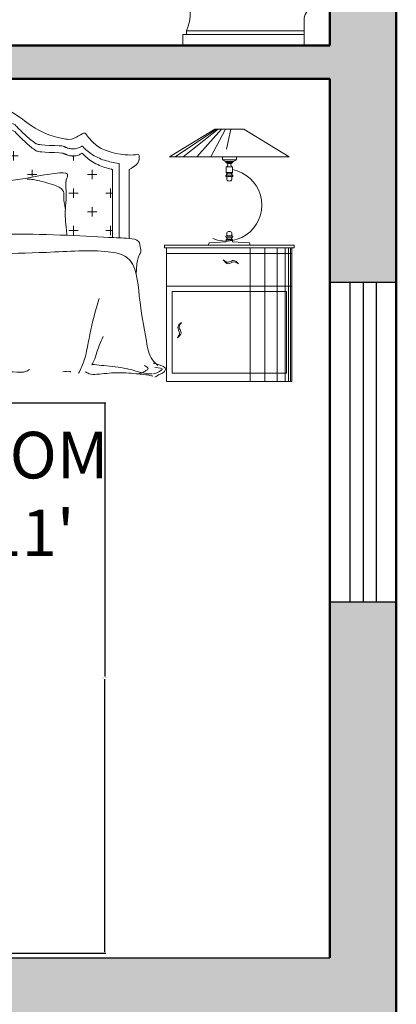
# Model space of a CAD drawing. Units: inches. Extents: x 1771 to 3025, y 319 to 889.
# Tile 17 of 35: x 2505 to 2561, y 473 to 621. Entities that reach past the tile are written whole.
import ezdxf

# ---------------------------------------------------------------- set-up
doc = ezdxf.new("R2010")
doc.units = ezdxf.units.IN
doc.header["$MEASUREMENT"] = 0
for name, color, linetype, lineweight in [('A-ANNO-DIMS', 2, 'Continuous', 18), ('A-AREA-IDEN', 241, 'Continuous', 25), ('A-FLOR-FIXT', 8, 'Continuous', 18), ('A-FLOR-STRS', 7, 'Continuous', 25), ('A-FURN', 8, 'Continuous', 18), ('A-GLAZ', 40, 'Continuous', 25), ('A-WALL', 7, 'Continuous', 50), ('A-WALL-PATT', 254, 'Continuous', 13)]:
    doc.layers.add(name, color=color, linetype=linetype, lineweight=lineweight)
doc.styles.get("Standard").update_dxf_attribs({"font": 'arial.ttf'})
doc.dimstyles.get("Standard").update_dxf_attribs({"dimtxt": 0.18, "dimasz": 0.18, "dimexe": 0.18, "dimexo": 0.0625, "dimgap": 0.09, "dimtad": 0, "dimtih": 1, "dimtoh": 1, "dimdec": 4, "dimzin": 0, "dimdsep": 46, "dimtxsty": 'Standard', "dimcen": 0.09, "dimadec": 0, "dimazin": 0, "dimtfac": 1, "dimtdec": 4, "dimtofl": 0, "dimtmove": 0, "dimatfit": 3, "dimfxl": 1, "dimtolj": 1, "dimtzin": 0, "dimarcsym": 0})

# ---------------------------------------------------------------- blocks, each defined once
blk = doc.blocks.new('A$C3908634B')
at = {"ltscale": 5}
for p, q in [((1200.2, 1046.3), (1218.1, 1046.3)), ((1176, 731), (1176, 731.7))]:
    blk.add_line(p, q, dxfattribs=at)
for p, q in [((1253.9, 945.1), (1253.9, 978.5)), ((1100.9, 962.2), (1134.6, 962.2)), ((1117.6, 945.1), (1117.6, 967.5)), ((1236.9, 962.2), (1271, 962.2)), ((184.3, 923.4), (19, 823.1)), ((237.5, 923.4), (184.3, 923.4)), ((190.2, 923.4), (237.5, 923.4)), ((231.9, 923.4), (247.3, 851.1)), ((284.7, 923.4), (237.5, 923.4)), ((237.5, 923.4), (290.6, 923.4)), ((251.7, 923.4), (305.7, 823.1)), ((266, 923.4), (356.4, 823.1)), ((278.7, 923.4), (406.8, 823.1)), ((284.7, 923.4), (436.3, 823.1)), ((290.6, 923.4), (456, 823.1)), ((1049.4, 876.9), (1049.4, 911)), ((1185.7, 876.9), (1185.7, 911)), ((1322.1, 876.9), (1322.1, 911)), ((2198.9, 923.4), (2033.5, 823.1)), ((2204.8, 923.4), (2053.3, 823.1)), ((2210.8, 923.4), (2082.7, 823.1)), ((2223.5, 923.4), (2133.1, 823.1)), ((2237.8, 923.4), (2183.8, 823.1)), ((2252, 923.4), (2198.9, 923.4)), ((2204.8, 923.4), (2252, 923.4)), ((2257.6, 923.4), (2242.2, 851.1)), ((2299.3, 923.4), (2252, 923.4)), ((2252, 923.4), (2305.2, 923.4)), ((2305.2, 923.4), (2470.5, 823.1)), ((1032.3, 894), (1066.4, 894)), ((1168.7, 894), (1202.8, 894)), ((1305.1, 894), (1339.1, 894)), ((940, 808.8), (940, 842.9)), ((1117.6, 808.8), (1117.6, 842.9)), ((1253.9, 808.8), (1253.9, 842.9)), ((1462.5, 808.8), (1462.5, 842.9)), ((237.5, 823.1), (19, 823.1)), ((212, 823.1), (212, 811.7)), ((212, 811.7), (223, 805.4)), ((212, 811.7), (237.5, 811.7)), ((223, 805.4), (224.6, 801.4)), ((223, 805.4), (237.5, 805.4)), ((250.4, 801.4), (224.6, 801.4)), ((226.9, 801.4), (228.3, 798.3)), ((228.3, 798.3), (237.5, 798.3)), ((228.3, 798.3), (231.3, 797.6)), ((231.3, 797.6), (232, 794.9)), ((231.9, 793.9), (231.6, 792.6)), ((232, 794.9), (231.9, 793.9)), ((237.5, 823.1), (456, 823.1)), ((263, 811.7), (237.5, 811.7)), ((252, 805.4), (237.5, 805.4)), ((246.7, 798.3), (237.5, 798.3)), ((243.7, 797.6), (243, 794.9)), ((243, 794.9), (243.1, 793.9)), ((243.1, 793.9), (243.4, 792.6)), ((246.7, 798.3), (243.7, 797.6)), ((248.1, 801.4), (246.7, 798.3)), ((252, 805.4), (250.4, 801.4)), ((263, 811.7), (252, 805.4)), ((263, 823.1), (263, 811.7)), ((621.3, 798.8), (621.3, 526)), ((741.7, 808.8), (741.7, 821.7)), ((746.2, 825.8), (758.8, 825.8)), ((922.9, 825.8), (957, 825.8)), ((1100.5, 825.8), (1134.6, 825.8)), ((1236.9, 825.8), (1271, 825.8)), ((1373.2, 825.8), (1479.5, 825.8)), ((1681.3, 808.8), (1681.3, 825.6)), ((1848.6, 798.8), (1848.6, 526.2)), ((2252, 823.1), (2033.5, 823.1)), ((2226.5, 823.1), (2226.5, 811.7)), ((2226.5, 811.7), (2237.6, 805.4)), ((2226.5, 811.7), (2252, 811.7)), ((2237.6, 805.4), (2239.1, 801.4)), ((2237.6, 805.4), (2252, 805.4)), ((2239.1, 801.4), (2264.9, 801.4)), ((2241.4, 801.4), (2242.8, 798.3)), ((2242.8, 798.3), (2245.8, 797.6)), ((2242.8, 798.3), (2252, 798.3)), ((2245.8, 797.6), (2246.5, 794.9)), ((2246.4, 793.9), (2246.1, 792.6)), ((2246.5, 794.9), (2246.4, 793.9)), ((2252, 823.1), (2470.5, 823.1)), ((2277.6, 811.7), (2252, 811.7)), ((2266.5, 805.4), (2252, 805.4)), ((2261.2, 798.3), (2252, 798.3)), ((2258.2, 797.6), (2257.6, 794.9)), ((2257.6, 794.9), (2257.6, 793.9)), ((2257.6, 793.9), (2257.9, 792.6)), ((2261.2, 798.3), (2258.2, 797.6)), ((2262.6, 801.4), (2261.2, 798.3)), ((2266.5, 805.4), (2264.9, 801.4)), ((2277.6, 811.7), (2266.5, 805.4)), ((2277.6, 823.1), (2277.6, 811.7)), ((227.8, 786.4), (226.2, 785.6)), ((226.2, 785.6), (226.2, 765)), ((226.2, 785.6), (248.8, 785.6)), ((226.2, 765), (227.6, 764.2)), ((226.2, 765), (237.5, 765)), ((227.4, 757.9), (227.1, 757.2)), ((227.1, 757.2), (227.3, 756.6)), ((227.3, 756.6), (227.8, 755.9)), ((227.7, 758.5), (227.4, 757.9)), ((227.6, 764.2), (228.5, 763.3)), ((228.6, 758.7), (227.7, 758.5)), ((230.2, 788), (227.8, 786.4)), ((228.5, 763.3), (229.4, 762.5)), ((228.5, 763.3), (237.5, 763.3)), ((229.4, 759.1), (228.6, 758.7)), ((229.4, 762.5), (230, 761.4)), ((229.8, 759.5), (229.4, 759.1)), ((230.1, 760.2), (229.8, 759.5)), ((230, 761.4), (230.1, 760.2)), ((231.1, 790.5), (230.2, 788)), ((231.5, 791.1), (231.1, 790.5)), ((231.6, 792.6), (231.5, 791.9)), ((231.5, 791.9), (231.5, 791.1)), ((248.8, 765), (237.5, 765)), ((246.5, 763.3), (237.5, 763.3)), ((243.4, 792.6), (243.4, 791.9)), ((243.4, 791.9), (243.4, 791.1)), ((243.4, 791.1), (243.9, 790.5)), ((243.9, 790.5), (244.8, 788)), ((244.8, 788), (247.2, 786.4)), ((245, 761.4), (244.9, 760.2)), ((244.9, 760.2), (245.2, 759.5)), ((245.6, 762.5), (245, 761.4)), ((245.2, 759.5), (245.6, 759.1)), ((246.5, 763.3), (245.6, 762.5)), ((245.6, 759.1), (246.4, 758.7)), ((246.4, 758.7), (247.3, 758.5)), ((247.4, 764.2), (246.5, 763.3)), ((247.2, 786.4), (248.8, 785.6)), ((247.7, 756.6), (247.2, 755.9)), ((247.3, 758.5), (247.6, 757.9)), ((248.8, 765), (247.4, 764.2)), ((247.6, 757.9), (247.9, 757.2)), ((247.9, 757.2), (247.7, 756.6)), ((248.8, 785.6), (248.8, 765)), ((645.8, 776.5), (645.8, 527)), ((656.5, 757.6), (690.6, 757.6)), ((673.5, 740.6), (673.5, 774.7)), ((792.9, 757.6), (827, 757.6)), ((809.9, 740.6), (809.9, 774.7)), ((1032.3, 757.6), (1066.4, 757.6)), ((1049.4, 740.6), (1049.4, 774.7)), ((1168.7, 757.6), (1202.8, 757.6)), ((1185.7, 740.6), (1185.7, 774.7)), ((1305.1, 757.6), (1339.1, 757.6)), ((1322.1, 740.6), (1322.1, 774.7)), ((1513.6, 757.6), (1547.7, 757.6)), ((1530.6, 751.3), (1530.6, 774.7)), ((1732.4, 757.6), (1766.5, 757.6)), ((1749.5, 740.6), (1749.5, 774.7)), ((1824, 776.5), (1824, 527.2)), ((2242.3, 786.4), (2240.7, 785.6)), ((2240.7, 785.6), (2240.7, 765)), ((2263.3, 785.6), (2240.7, 785.6)), ((2240.7, 765), (2242.1, 764.2)), ((2240.7, 765), (2252, 765)), ((2241.9, 757.9), (2241.7, 757.2)), ((2241.7, 757.2), (2241.8, 756.6)), ((2241.8, 756.6), (2242.3, 755.9)), ((2242.2, 758.5), (2241.9, 757.9)), ((2242.1, 764.2), (2243, 763.3)), ((2243.1, 758.7), (2242.2, 758.5)), ((2244.7, 788), (2242.3, 786.4)), ((2243, 763.3), (2243.9, 762.5)), ((2243, 763.3), (2252, 763.3)), ((2243.9, 759.1), (2243.1, 758.7)), ((2243.9, 762.5), (2244.6, 761.4)), ((2244.3, 759.5), (2243.9, 759.1)), ((2244.6, 760.2), (2244.3, 759.5)), ((2244.6, 761.4), (2244.6, 760.2)), ((2245.6, 790.5), (2244.7, 788)), ((2246.1, 791.1), (2245.6, 790.5)), ((2246.1, 792.6), (2246.1, 791.9)), ((2246.1, 791.9), (2246.1, 791.1)), ((2263.3, 765), (2252, 765)), ((2261.1, 763.3), (2252, 763.3)), ((2257.9, 792.6), (2258, 791.9)), ((2258, 791.9), (2258, 791.1)), ((2258, 791.1), (2258.4, 790.5)), ((2258.4, 790.5), (2259.4, 788)), ((2259.4, 788), (2261.7, 786.4)), ((2259.5, 761.4), (2259.4, 760.2)), ((2259.4, 760.2), (2259.7, 759.5)), ((2260.1, 762.5), (2259.5, 761.4)), ((2259.7, 759.5), (2260.1, 759.1)), ((2261.1, 763.3), (2260.1, 762.5)), ((2260.1, 759.1), (2260.9, 758.7)), ((2260.9, 758.7), (2261.8, 758.5)), ((2261.9, 764.2), (2261.1, 763.3)), ((2261.7, 786.4), (2263.3, 785.6)), ((2261.8, 758.5), (2262.2, 757.9)), ((2262.2, 756.6), (2261.8, 755.9)), ((2263.3, 765), (2261.9, 764.2)), ((2262.2, 757.9), (2262.4, 757.2)), ((2262.4, 757.2), (2262.2, 756.6)), ((2263.3, 785.6), (2263.3, 765)), ((224.8, 753.5), (224.7, 752.9)), ((224.7, 752.9), (224.8, 752.1)), ((225.3, 753.9), (224.8, 753.5)), ((224.8, 752.1), (225.2, 751.4)), ((225.2, 751.4), (225.6, 750.9)), ((225.7, 754.3), (225.3, 753.9)), ((225.6, 750.9), (228.1, 750.2)), ((226.3, 754.6), (225.7, 754.3)), ((227, 754.7), (226.3, 754.6)), ((227.9, 754.7), (227, 754.7)), ((227.8, 755.9), (228.9, 755.2)), ((228.9, 755.2), (227.9, 754.7)), ((228.1, 750.2), (229.9, 750)), ((228.9, 755.2), (237.5, 755.2)), ((229.9, 750), (232.4, 750.2)), ((232.4, 750.2), (237.5, 750.2)), ((246.1, 755.2), (237.5, 755.2)), ((242.6, 750.2), (237.5, 750.2)), ((245.1, 750), (242.6, 750.2)), ((246.9, 750.2), (245.1, 750)), ((247.2, 755.9), (246.1, 755.2)), ((246.1, 755.2), (247.1, 754.7)), ((249.4, 750.9), (246.9, 750.2)), ((247.1, 754.7), (248, 754.7)), ((248, 754.7), (248.7, 754.6)), ((248.7, 754.6), (249.3, 754.3)), ((249.3, 754.3), (249.7, 753.9)), ((249.8, 751.4), (249.4, 750.9)), ((249.7, 753.9), (250.2, 753.5)), ((250.2, 752.1), (249.8, 751.4)), ((250.2, 753.5), (250.3, 752.9)), ((250.3, 752.9), (250.2, 752.1)), ((2239.4, 753.5), (2239.2, 752.9)), ((2239.2, 752.9), (2239.3, 752.1)), ((2239.3, 752.1), (2239.7, 751.4)), ((2239.9, 753.9), (2239.4, 753.5)), ((2239.7, 751.4), (2240.2, 750.9)), ((2240.3, 754.3), (2239.9, 753.9)), ((2240.2, 750.9), (2242.6, 750.2)), ((2240.8, 754.6), (2240.3, 754.3)), ((2241.5, 754.7), (2240.8, 754.6)), ((2242.4, 754.7), (2241.5, 754.7)), ((2242.3, 755.9), (2243.4, 755.2)), ((2243.4, 755.2), (2242.4, 754.7)), ((2242.6, 750.2), (2244.4, 750)), ((2243.4, 755.2), (2252, 755.2)), ((2244.4, 750), (2246.9, 750.2)), ((2246.9, 750.2), (2252, 750.2)), ((2260.7, 755.2), (2252, 755.2)), ((2257.1, 750.2), (2252, 750.2)), ((2259.6, 750), (2257.1, 750.2)), ((2261.5, 750.2), (2259.6, 750)), ((2261.8, 755.9), (2260.7, 755.2)), ((2260.7, 755.2), (2261.6, 754.7)), ((2263.9, 750.9), (2261.5, 750.2)), ((2261.6, 754.7), (2262.5, 754.7)), ((2262.5, 754.7), (2263.2, 754.6)), ((2263.2, 754.6), (2263.8, 754.3)), ((2263.8, 754.3), (2264.2, 753.9)), ((2264.3, 751.4), (2263.9, 750.9)), ((2264.2, 753.9), (2264.7, 753.5)), ((2264.7, 752.1), (2264.3, 751.4)), ((2264.7, 753.5), (2264.8, 752.9)), ((2264.8, 752.9), (2264.7, 752.1)), ((724.7, 689.4), (758.8, 689.4)), ((741.7, 672.4), (741.7, 706.5)), ((922.9, 689.4), (957, 689.4)), ((940, 672.4), (940, 706.5)), ((1100.5, 689.4), (1134.6, 689.4)), ((1117.6, 672.4), (1117.6, 706.5)), ((1664.3, 689.4), (1698.3, 689.4)), ((1681.3, 672.4), (1681.3, 706.5)), ((1800.6, 689.4), (1824, 689.4)), ((1817.7, 672.4), (1817.7, 706.5)), ((656.5, 621.3), (690.6, 621.3)), ((673.5, 604.2), (673.5, 638.3)), ((792.9, 621.3), (823.2, 621.3)), ((809.9, 604.2), (809.9, 638.3)), ((1732.4, 621.3), (1766.5, 621.3)), ((1749.5, 604.2), (1749.5, 638.3)), ((724.7, 553.1), (758.8, 553.1)), ((741.7, 536), (741.7, 570.1)), ((1664.3, 553.1), (1698.3, 553.1)), ((1681.3, 536), (1681.3, 570.1)), ((1800.6, 553.1), (1824, 553.1)), ((1817.7, 536), (1817.7, 570.1)), ((164, 507.9), (161.1, 499.5)), ((164, 507.9), (226.2, 512.1)), ((224.7, 530.9), (224.8, 531.7)), ((224.8, 530.3), (224.7, 530.9)), ((224.8, 531.7), (225.2, 532.4)), ((225.3, 529.9), (224.8, 530.3)), ((225.2, 532.4), (225.6, 532.9)), ((225.7, 529.5), (225.3, 529.9)), ((225.6, 532.9), (228.1, 533.6)), ((226.3, 529.2), (225.7, 529.5)), ((226.2, 518.8), (227.6, 519.6)), ((226.2, 512.1), (226.2, 518.8)), ((226.2, 518.8), (237.5, 518.8)), ((227, 529.1), (226.3, 529.2)), ((227.9, 529.1), (227, 529.1)), ((227.1, 526.6), (227.3, 527.2)), ((227.4, 525.9), (227.1, 526.6)), ((227.3, 527.2), (227.8, 527.9)), ((227.7, 525.3), (227.4, 525.9)), ((227.6, 519.6), (228.5, 520.5)), ((228.6, 525.1), (227.7, 525.3)), ((227.8, 527.9), (228.9, 528.6)), ((228.9, 528.6), (227.9, 529.1)), ((228.1, 533.6), (229.9, 533.8)), ((228.5, 520.5), (229.4, 521.3)), ((229.4, 524.7), (228.6, 525.1)), ((228.9, 528.6), (237.5, 528.6)), ((229.8, 524.3), (229.4, 524.7)), ((229.4, 521.3), (230, 522.4)), ((229.4, 521.3), (237.5, 521.3)), ((230.1, 523.6), (229.8, 524.3)), ((230, 522.4), (230.1, 523.6)), ((230.3, 533.8), (237.5, 533.6)), ((242.6, 533.6), (237.5, 533.6)), ((246.1, 528.6), (237.5, 528.6)), ((245.6, 521.3), (237.5, 521.3)), ((248.8, 518.8), (237.5, 518.8)), ((245.1, 533.8), (242.6, 533.6)), ((244.9, 523.6), (245.2, 524.3)), ((245, 522.4), (244.9, 523.6)), ((245.6, 521.3), (245, 522.4)), ((246.9, 533.6), (245.1, 533.8)), ((245.2, 524.3), (245.6, 524.7)), ((245.6, 524.7), (246.4, 525.1)), ((246.5, 520.5), (245.6, 521.3)), ((246.1, 528.6), (247.1, 529.1)), ((247.2, 527.9), (246.1, 528.6)), ((246.4, 525.1), (247.3, 525.3)), ((247.4, 519.6), (246.5, 520.5)), ((249.4, 532.9), (246.9, 533.6)), ((247.1, 529.1), (248, 529.1)), ((247.7, 527.2), (247.2, 527.9)), ((247.3, 525.3), (247.6, 525.9)), ((248.8, 518.8), (247.4, 519.6)), ((247.6, 525.9), (247.9, 526.6)), ((247.9, 526.6), (247.7, 527.2)), ((248, 529.1), (248.7, 529.2)), ((248.7, 529.2), (249.3, 529.5)), ((248.8, 512.1), (248.8, 518.8)), ((311, 507.9), (248.8, 512.1)), ((249.3, 529.5), (249.7, 529.9)), ((249.8, 532.4), (249.4, 532.9)), ((249.7, 529.9), (250.2, 530.3)), ((250.2, 531.7), (249.8, 532.4)), ((250.3, 530.9), (250.2, 531.7)), ((250.2, 530.3), (250.3, 530.9)), ((311, 507.9), (315.3, 499.5)), ((2178.5, 507.9), (2174.2, 499.5)), ((2178.5, 507.9), (2240.7, 512.1)), ((2239.2, 530.9), (2239.3, 531.7)), ((2239.4, 530.3), (2239.2, 530.9)), ((2239.3, 531.7), (2239.7, 532.4)), ((2239.9, 529.9), (2239.4, 530.3)), ((2239.7, 532.4), (2240.2, 532.9)), ((2240.3, 529.5), (2239.9, 529.9)), ((2240.2, 532.9), (2242.6, 533.6)), ((2240.8, 529.2), (2240.3, 529.5)), ((2240.7, 518.8), (2242.1, 519.6)), ((2240.7, 512.1), (2240.7, 518.8)), ((2240.7, 518.8), (2252, 518.8)), ((2241.5, 529.1), (2240.8, 529.2)), ((2242.4, 529.1), (2241.5, 529.1)), ((2241.7, 526.6), (2241.8, 527.2)), ((2241.9, 525.9), (2241.7, 526.6)), ((2241.8, 527.2), (2242.3, 527.9)), ((2242.2, 525.3), (2241.9, 525.9)), ((2242.1, 519.6), (2243, 520.5)), ((2243.1, 525.1), (2242.2, 525.3)), ((2242.3, 527.9), (2243.4, 528.6)), ((2243.4, 528.6), (2242.4, 529.1)), ((2242.6, 533.6), (2244.4, 533.8)), ((2243, 520.5), (2243.9, 521.3)), ((2243.9, 524.7), (2243.1, 525.1)), ((2243.4, 528.6), (2252, 528.6)), ((2244.3, 524.3), (2243.9, 524.7)), ((2243.9, 521.3), (2244.6, 522.4)), ((2243.9, 521.3), (2252, 521.3)), ((2244.6, 523.6), (2244.3, 524.3)), ((2244.4, 533.8), (2246.9, 533.6)), ((2244.6, 522.4), (2244.6, 523.6)), ((2246.9, 533.6), (2252, 533.6)), ((2259.2, 533.8), (2252, 533.6)), ((2260.7, 528.6), (2252, 528.6)), ((2260.1, 521.3), (2252, 521.3)), ((2263.3, 518.8), (2252, 518.8)), ((2259.4, 523.6), (2259.7, 524.3)), ((2259.5, 522.4), (2259.4, 523.6)), ((2260.1, 521.3), (2259.5, 522.4)), ((2261.5, 533.6), (2259.6, 533.8)), ((2259.7, 524.3), (2260.1, 524.7)), ((2260.1, 524.7), (2260.9, 525.1)), ((2261.1, 520.5), (2260.1, 521.3)), ((2260.7, 528.6), (2261.6, 529.1)), ((2261.8, 527.9), (2260.7, 528.6)), ((2260.9, 525.1), (2261.8, 525.3)), ((2261.9, 519.6), (2261.1, 520.5)), ((2263.9, 532.9), (2261.5, 533.6)), ((2261.6, 529.1), (2262.5, 529.1)), ((2262.2, 527.2), (2261.8, 527.9)), ((2261.8, 525.3), (2262.2, 525.9)), ((2263.3, 518.8), (2261.9, 519.6)), ((2262.4, 526.6), (2262.2, 527.2)), ((2262.2, 525.9), (2262.4, 526.6)), ((2262.5, 529.1), (2263.2, 529.2)), ((2263.2, 529.2), (2263.8, 529.5)), ((2263.3, 512.1), (2263.3, 518.8)), ((2325.5, 507.9), (2263.3, 512.1)), ((2263.8, 529.5), (2264.2, 529.9)), ((2264.3, 532.4), (2263.9, 532.9)), ((2264.2, 529.9), (2264.7, 530.3)), ((2264.7, 531.7), (2264.3, 532.4)), ((2264.8, 530.9), (2264.7, 531.7)), ((2264.7, 530.3), (2264.8, 530.9)), ((2325.5, 507.9), (2328.4, 499.5)), ((475, 499.5), (0, 499.5)), ((0, 499.5), (0, 489.5)), ((475, 489.5), (0, 489.5)), ((8.7, 489.5), (8.7, 0)), ((467.1, 469.5), (8.7, 469.5)), ((14.1, 488.6), (14.1, 0)), ((21.3, 488.6), (21.3, 0)), ((33, 488.6), (33, 0)), ((62.7, 488.6), (62.7, 0)), ((107.6, 488.6), (107.6, 0)), ((161.1, 499.5), (237.5, 499.5)), ((161.6, 488.6), (161.6, 0)), ((315.3, 499.5), (237.5, 499.5)), ((467.1, 0), (467.1, 489.5)), ((475, 499.5), (475, 489.5)), ((2014.5, 499.5), (2489.5, 499.5)), ((2014.5, 499.5), (2014.5, 489.5)), ((2014.5, 489.5), (2489.5, 489.5)), ((2022.4, 0), (2022.4, 489.5)), ((2022.4, 469.5), (2480.8, 469.5)), ((2174.2, 499.5), (2252, 499.5)), ((2328.4, 499.5), (2252, 499.5)), ((2327.9, 488.6), (2327.9, 0)), ((2381.9, 488.6), (2381.9, 0)), ((2426.8, 488.6), (2426.8, 0)), ((2456.5, 488.6), (2456.5, 0)), ((2468.2, 488.6), (2468.2, 0)), ((2475.4, 488.6), (2475.4, 0)), ((2480.8, 489.5), (2480.8, 0)), ((2489.5, 499.5), (2489.5, 489.5)), ((467.1, 349.5), (8.7, 349.5)), ((28.7, 329.5), (28.7, 31.6)), ((447.1, 329.5), (28.7, 329.5)), ((447.1, 31.6), (447.1, 329.5)), ((2022.4, 349.5), (2480.8, 349.5)), ((2042.4, 329.5), (2460.8, 329.5)), ((2042.4, 31.6), (2042.4, 329.5)), ((2460.8, 329.5), (2460.8, 31.6)), ((467.1, 281.6), (467.1, 301.6)), ((2022.4, 281.6), (2022.4, 301.6)), ((8.7, 0), (467.1, 0)), ((28.7, 31.6), (447.1, 31.6)), ((2022.4, 0), (2480.8, 0)), ((2460.8, 31.6), (2042.4, 31.6))]:
    blk.add_line(p, q)
at = {"ltscale": 20}
for p, q in [((584.4, 776.7), (584.4, 523.7)), ((1885.4, 776.7), (1885.4, 524))]:
    blk.add_line(p, q, dxfattribs=at)
for centre, radius, start, end in [((1209.1, 956.2), 55.2, 80.5605, 99.4395), ((1209.1, 930.3), 55.2, 80.5605, 99.4395), ((250.5, 646.2), 131.8, 100.6234, 291.2), ((2239, 646.2), 131.8, 248.8, 79.3766), ((237.5, 743.5), 9.69, 137.7341, 270), ((237.5, 743.5), 9.69, 270, 42.2659), ((2252, 743.5), 9.69, 137.7341, 270), ((2252, 743.5), 9.69, 270, 42.2659), ((237.5, 540.3), 9.69, 90, 222.2659), ((237.5, 540.3), 9.69, 317.7341, 90), ((2252, 540.3), 9.69, 90, 222.2659), ((2252, 540.3), 9.69, 317.7341, 90)]:
    blk.add_arc(centre, radius, start, end)
for points in [[(584.4, 776.7), (563.9, 786.2), (546, 802.1), (547.3, 834.8), (564.5, 828.3), (620.6, 830.4), (706.4, 847.2), (752.1, 924.2), (778.1, 880.4), (846.1, 907.1), (1017.7, 1014.1), (1134.5, 1035.5), (1200.2, 1046.3)], [(1885.4, 776.7), (1905.9, 786.2), (1923.9, 802.1), (1922.5, 834.8), (1905.3, 828.3), (1849.2, 830.4), (1763.4, 847.2), (1717.7, 924.2), (1691.7, 880.4), (1541.2, 907.1), (1472.8, 1014.1), (1283.8, 1035.5), (1218.1, 1046.3)]]:
    blk.add_open_spline(points, degree=3, knots=[12.417853, 12.417853, 12.417853, 12.417853, 68.394536, 90.665986, 114.156853, 157.554067, 281.869614, 298.858744, 338.737111, 347.060176, 470.423438, 625.498764, 625.498764, 625.498764, 625.498764], dxfattribs=at)
for points, knots in [([(756.1, 861.8), (756.9, 861.3), (757.6, 860.9), (759.9, 859.6), (761.6, 858.7), (765.5, 856.8), (767.8, 855.8), (772.7, 854.1), (775.4, 853.3), (780.8, 852.2), (783.3, 851.8), (787.1, 851.6), (788.2, 851.5), (789.9, 851.5), (790.6, 851.5), (791.9, 851.5), (792.5, 851.5), (793.6, 851.6), (794.1, 851.6), (795.8, 851.8), (796.8, 851.9), (800.3, 852.3), (802.5, 852.8), (806.5, 853.8), (808.3, 854.3), (811.5, 855.4), (812.9, 855.9), (815.3, 856.9), (816.4, 857.4), (817.6, 857.9), (817.8, 858), (818.4, 858.2), (818.7, 858.4), (819.5, 858.7), (820, 859), (821.6, 859.7), (822.7, 860.2), (825.8, 861.7), (827.9, 862.8), (834, 866), (837.9, 868.3), (848.5, 874.9), (854.9, 879.4), (928.8, 888.8), (934.4, 893.5), (945, 903.2), (950, 908), (1000.9, 917.4), (1005.5, 922.1), (1014.4, 931), (1018.7, 935.3), (1027, 943.5), (1031.1, 947.3), (1036.9, 952.4), (1038.8, 954), (1042, 956.7), (1043.5, 957.9), (1045.8, 959.7), (1046.7, 960.3), (1048.5, 961.7), (1049.4, 962.3), (1052.1, 964.2), (1054, 965.5), (1059.7, 969.2), (1063.6, 971.5), (1074.8, 977.5), (1082.2, 980.9), (1098, 987.2), (1106.3, 990), (1123.7, 995.2), (1132.8, 997.5), (1151.5, 1001.8), (1161.1, 1003.8), (1180.5, 1007.4), (1190.2, 1009), (1200.1, 1010.7)], [328.6705, 328.6705, 328.6705, 328.6705, 329.609368, 329.609368, 331.487103, 331.487103, 333.620342, 333.620342, 335.753581, 335.753581, 337.507866, 337.507866, 338.182373, 338.182373, 338.607397, 338.607397, 338.959312, 338.959312, 339.311227, 339.311227, 340.015058, 340.015058, 341.722742, 341.722742, 343.430427, 343.430427, 345.138111, 345.138111, 346.845796, 346.845796, 347.37881, 347.37881, 347.911824, 347.911824, 348.977853, 348.977853, 351.109909, 351.109909, 355.374023, 355.374023, 363.902249, 363.902249, 379.258481, 379.258481, 394.614712, 394.614712, 409.970944, 409.970944, 425.327175, 425.327175, 440.683406, 440.683406, 456.039638, 456.039638, 463.285514, 463.285514, 469.01116, 469.01116, 472.593, 472.593, 476.17484, 476.17484, 483.338521, 483.338521, 497.665882, 497.665882, 522.309302, 522.309302, 546.952723, 546.952723, 571.596143, 571.596143, 596.239564, 596.239564, 619.876409, 619.876409, 619.876409, 619.876409]), ([(1713.7, 861.8), (1713, 861.3), (1712.2, 860.9), (1709.9, 859.6), (1708.2, 858.7), (1704.3, 856.8), (1702.1, 855.8), (1697.1, 854.1), (1694.4, 853.3), (1689.1, 852.2), (1686.5, 851.8), (1682.7, 851.6), (1681.7, 851.5), (1679.9, 851.5), (1679.2, 851.5), (1678, 851.5), (1677.4, 851.5), (1676.2, 851.6), (1675.7, 851.6), (1674.1, 851.8), (1673, 851.9), (1669.5, 852.3), (1667.3, 852.8), (1663.3, 853.8), (1661.5, 854.3), (1658.4, 855.4), (1657, 855.9), (1654.5, 856.9), (1653.4, 857.4), (1652.2, 857.9), (1652, 858), (1651.4, 858.2), (1651.2, 858.4), (1650.4, 858.7), (1649.8, 859), (1648.2, 859.7), (1647.1, 860.2), (1644, 861.7), (1641.9, 862.8), (1553.3, 866), (1549.4, 868.3), (1538.8, 874.9), (1532.4, 879.4), (1520.4, 888.8), (1514.8, 893.5), (1504.2, 903.2), (1499.2, 908), (1489.5, 917.4), (1484.9, 922.1), (1476.1, 931), (1471.8, 935.3), (1463.4, 943.5), (1459.4, 947.3), (1381.4, 952.4), (1379.5, 954), (1376.2, 956.7), (1374.8, 957.9), (1372.5, 959.7), (1371.6, 960.3), (1369.8, 961.7), (1368.9, 962.3), (1366.2, 964.2), (1364.3, 965.5), (1358.6, 969.2), (1354.6, 971.5), (1343.5, 977.5), (1336, 980.9), (1320.2, 987.2), (1311.9, 990), (1294.6, 995.2), (1285.5, 997.5), (1266.8, 1001.8), (1257.2, 1003.8), (1237.8, 1007.4), (1228.1, 1009), (1218.2, 1010.7)], [328.6705, 328.6705, 328.6705, 328.6705, 329.609368, 329.609368, 331.487103, 331.487103, 333.620342, 333.620342, 335.753581, 335.753581, 337.507866, 337.507866, 338.182373, 338.182373, 338.607397, 338.607397, 338.959312, 338.959312, 339.311227, 339.311227, 340.015058, 340.015058, 341.722742, 341.722742, 343.430427, 343.430427, 345.138111, 345.138111, 346.845796, 346.845796, 347.37881, 347.37881, 347.911824, 347.911824, 348.977853, 348.977853, 351.109909, 351.109909, 355.374023, 355.374023, 363.902249, 363.902249, 379.258481, 379.258481, 394.614712, 394.614712, 409.970943, 409.970943, 425.327175, 425.327175, 440.683406, 440.683406, 456.039637, 456.039637, 463.285514, 463.285514, 469.011154, 469.011154, 472.592992, 472.592992, 476.17483, 476.17483, 483.338506, 483.338506, 497.665857, 497.665857, 522.309275, 522.309275, 546.952693, 546.952693, 571.59611, 571.59611, 596.239528, 596.239528, 619.876409, 619.876409, 619.876409, 619.876409]), ([(756.1, 835.9), (756.9, 835.5), (757.6, 835), (759.9, 833.7), (761.6, 832.8), (765.5, 830.9), (767.8, 830), (772.7, 828.2), (775.4, 827.5), (780.8, 826.3), (783.3, 826), (787.1, 825.7), (788.2, 825.7), (789.9, 825.6), (790.6, 825.6), (791.9, 825.6), (792.5, 825.7), (793.6, 825.7), (794.1, 825.8), (795.8, 825.9), (796.8, 826), (800.3, 826.5), (802.5, 826.9), (806.5, 827.9), (808.3, 828.5), (811.5, 829.5), (812.9, 830.1), (815.3, 831), (816.4, 831.5), (817.6, 832), (817.8, 832.1), (818.4, 832.4), (818.7, 832.5), (819.5, 832.9), (820, 833.1), (821.6, 833.8), (822.7, 834.3), (825.8, 835.9), (827.9, 836.9), (834, 840.2), (837.9, 842.4), (848.5, 849), (854.9, 853.6), (928.8, 862.9), (934.4, 867.7), (945, 877.3), (950, 882.1), (1000.9, 891.6), (1005.5, 896.2), (1014.4, 905.2), (1018.7, 909.5), (1027, 917.6), (1031.1, 921.4), (1036.9, 926.6), (1038.8, 928.2), (1042, 930.9), (1043.5, 932), (1045.8, 933.8), (1046.7, 934.5), (1048.5, 935.8), (1049.4, 936.4), (1052.1, 938.4), (1054, 939.6), (1059.7, 943.3), (1063.6, 945.6), (1074.8, 951.6), (1082.2, 955), (1098, 961.3), (1106.3, 964.2), (1123.7, 969.3), (1132.8, 971.6), (1151.5, 975.9), (1161.1, 977.9), (1180.5, 981.5), (1190.2, 983.2), (1200.1, 984.8)], [328.6705, 328.6705, 328.6705, 328.6705, 329.609368, 329.609368, 331.487103, 331.487103, 333.620342, 333.620342, 335.753581, 335.753581, 337.507866, 337.507866, 338.182373, 338.182373, 338.607397, 338.607397, 338.959312, 338.959312, 339.311227, 339.311227, 340.015058, 340.015058, 341.722742, 341.722742, 343.430427, 343.430427, 345.138111, 345.138111, 346.845796, 346.845796, 347.37881, 347.37881, 347.911824, 347.911824, 348.977853, 348.977853, 351.109909, 351.109909, 355.374023, 355.374023, 363.902249, 363.902249, 379.258481, 379.258481, 394.614712, 394.614712, 409.970944, 409.970944, 425.327175, 425.327175, 440.683406, 440.683406, 456.039638, 456.039638, 463.285514, 463.285514, 469.01116, 469.01116, 472.593, 472.593, 476.17484, 476.17484, 483.338521, 483.338521, 497.665882, 497.665882, 522.309302, 522.309302, 546.952723, 546.952723, 571.596143, 571.596143, 596.239564, 596.239564, 619.876409, 619.876409, 619.876409, 619.876409]), ([(1713.7, 835.9), (1713, 835.5), (1712.2, 835), (1709.9, 833.7), (1708.2, 832.8), (1704.3, 830.9), (1702.1, 830), (1697.1, 828.2), (1694.4, 827.5), (1689.1, 826.3), (1686.5, 826), (1682.7, 825.7), (1681.7, 825.7), (1679.9, 825.6), (1679.2, 825.6), (1678, 825.6), (1677.4, 825.7), (1676.2, 825.7), (1675.7, 825.8), (1674.1, 825.9), (1673, 826), (1669.5, 826.5), (1667.3, 826.9), (1663.3, 827.9), (1661.5, 828.5), (1658.4, 829.5), (1657, 830.1), (1654.5, 831), (1653.4, 831.5), (1652.2, 832), (1652, 832.1), (1651.4, 832.4), (1651.2, 832.5), (1650.4, 832.9), (1649.8, 833.1), (1648.2, 833.8), (1647.1, 834.3), (1644, 835.9), (1641.9, 836.9), (1553.3, 840.2), (1549.4, 842.4), (1538.8, 849), (1532.4, 853.6), (1520.4, 862.9), (1514.8, 867.7), (1504.2, 877.3), (1499.2, 882.1), (1489.5, 891.6), (1484.9, 896.2), (1476.1, 905.2), (1471.8, 909.5), (1463.4, 917.6), (1459.4, 921.4), (1381.4, 926.6), (1379.5, 928.2), (1376.2, 930.9), (1374.8, 932), (1372.5, 933.8), (1371.6, 934.5), (1369.8, 935.8), (1368.9, 936.4), (1366.2, 938.4), (1364.3, 939.6), (1358.6, 943.3), (1354.6, 945.6), (1343.5, 951.6), (1336, 955), (1320.2, 961.3), (1311.9, 964.2), (1294.6, 969.3), (1285.5, 971.6), (1266.8, 975.9), (1257.2, 977.9), (1237.8, 981.5), (1228.1, 983.2), (1218.2, 984.8)], [328.6705, 328.6705, 328.6705, 328.6705, 329.609368, 329.609368, 331.487103, 331.487103, 333.620342, 333.620342, 335.753581, 335.753581, 337.507866, 337.507866, 338.182373, 338.182373, 338.607397, 338.607397, 338.959312, 338.959312, 339.311227, 339.311227, 340.015058, 340.015058, 341.722742, 341.722742, 343.430427, 343.430427, 345.138111, 345.138111, 346.845796, 346.845796, 347.37881, 347.37881, 347.911824, 347.911824, 348.977853, 348.977853, 351.109909, 351.109909, 355.374023, 355.374023, 363.902249, 363.902249, 379.258481, 379.258481, 394.614712, 394.614712, 409.970943, 409.970943, 425.327175, 425.327175, 440.683406, 440.683406, 456.039637, 456.039637, 463.285514, 463.285514, 469.011154, 469.011154, 472.592992, 472.592992, 476.17483, 476.17483, 483.338506, 483.338506, 497.665857, 497.665857, 522.309275, 522.309275, 546.952693, 546.952693, 571.59611, 571.59611, 596.239528, 596.239528, 619.876409, 619.876409, 619.876409, 619.876409]), ([(621.3, 798.8), (633.4, 799.9), (641.2, 801.3), (657.3, 805), (665.7, 807.2), (682.6, 812.8), (691.1, 816.1), (708.1, 824.2), (716.5, 828.9), (731.3, 839), (737.9, 844.1), (748.3, 853.5), (752.3, 857.5), (756.1, 861.8)], [179.330708, 179.330708, 179.330708, 179.330708, 196.086144, 196.086144, 213.445516, 213.445516, 230.804888, 230.804888, 248.16426, 248.16426, 262.451931, 262.451931, 271.832526, 271.832526, 271.832526, 271.832526]), ([(645.8, 776.5), (646.9, 776.7), (648, 777), (657.3, 779.1), (665.7, 781.3), (682.6, 786.9), (691.1, 790.3), (708.1, 798.3), (716.5, 803), (731.3, 813.1), (737.9, 818.2), (748.3, 827.7), (752.3, 831.7), (756.1, 835.9)], [193.740688, 193.740688, 193.740688, 193.740688, 196.086144, 196.086144, 213.445516, 213.445516, 230.804888, 230.804888, 248.16426, 248.16426, 262.451931, 262.451931, 271.832526, 271.832526, 271.832526, 271.832526]), ([(1848.6, 798.8), (1836.4, 799.9), (1828.6, 801.3), (1812.5, 805), (1804.1, 807.2), (1787.2, 812.8), (1778.7, 816.1), (1761.8, 824.2), (1753.4, 828.9), (1738.5, 839), (1731.9, 844.1), (1721.5, 853.5), (1717.5, 857.5), (1713.7, 861.8)], [179.400376, 179.400376, 179.400376, 179.400376, 196.086144, 196.086144, 213.445516, 213.445516, 230.804888, 230.804888, 248.16426, 248.16426, 262.451931, 262.451931, 271.832526, 271.832526, 271.832526, 271.832526]), ([(1824, 776.5), (1822.9, 776.7), (1821.8, 777), (1812.5, 779.1), (1804.1, 781.3), (1787.2, 786.9), (1778.7, 790.3), (1761.8, 798.3), (1753.4, 803), (1738.5, 813.1), (1731.9, 818.2), (1721.5, 827.7), (1717.5, 831.7), (1713.7, 835.9)], [193.740688, 193.740688, 193.740688, 193.740688, 196.086144, 196.086144, 213.445516, 213.445516, 230.804888, 230.804888, 248.16426, 248.16426, 262.451931, 262.451931, 271.832526, 271.832526, 271.832526, 271.832526]), ([(1181.8, 730.2), (1176.9, 727.3), (1167.9, 723.5), (1152.3, 726.4), (1145.2, 713.6), (1142.1, 705.5), (1140.6, 701.2)], [16.588235, 16.588235, 16.588235, 16.588235, 39.368234, 56.465167, 72.647278, 91.317886, 91.317886, 91.317886, 91.317886]), ([(1512.2, 740.7), (1519.9, 740.7), (1533.1, 740.8), (1553.9, 735.5), (1652.4, 710.7), (1643.1, 675.3), (1648.8, 648.1), (1651.8, 634.5), (1651.9, 634)], [0, 0, 0, 0, 31.268494, 53.71641, 83.24833, 138.583941, 192.96698, 194.695488, 194.695488, 194.695488, 194.695488]), ([(1167.2, 686.5), (1175.5, 684.3), (1192.8, 677.8), (1196.3, 659.6), (1197.1, 648.3)], [13.535772, 13.535772, 13.535772, 13.535772, 45.871957, 87.312392, 87.312392, 87.312392, 87.312392]), ([(849.2, 653.1), (844.3, 648.8), (832.7, 636.7), (919.4, 609.9), (841.8, 577.9), (927.1, 550.1), (918.1, 541), (854.7, 539.8)], [5.952535, 5.952535, 5.952535, 5.952535, 29.258845, 70.114919, 115.518645, 162.322231, 169.813565, 169.813565, 169.813565, 169.813565]), ([(259.6, 445.5), (254.3, 441.1), (244.8, 433.2), (231.9, 440.9), (217, 446), (209.2, 437.1), (203.4, 430.5)], [0, 0, 0, 0, 18.381528, 32.980054, 40.875646, 63.595153, 63.595153, 63.595153, 63.595153]), ([(259.6, 445.5), (254, 438.6), (242.8, 424.9), (221, 442.9), (208.9, 434.4), (203.4, 430.5)], [0, 0, 0, 0, 22.772447, 45.052082, 63.466582, 63.466582, 63.466582, 63.466582]), ([(2229.9, 445.5), (2235.6, 438.6), (2246.7, 424.9), (2268.5, 442.9), (2280.6, 434.4), (2286.1, 430.5)], [0, 0, 0, 0, 22.772447, 45.052082, 63.466582, 63.466582, 63.466582, 63.466582]), ([(2229.9, 445.5), (2235.2, 441.1), (2244.7, 433.2), (2257.6, 440.9), (2272.5, 446), (2280.3, 437.1), (2286.1, 430.5)], [0, 0, 0, 0, 18.381528, 32.980054, 40.875646, 63.595153, 63.595153, 63.595153, 63.595153]), ([(412.3, 216.6), (419.2, 211), (432.8, 199.9), (414.9, 178.1), (423.4, 166), (427.2, 160.5)], [0, 0, 0, 0, 22.772447, 45.052082, 63.466582, 63.466582, 63.466582, 63.466582]), ([(412.3, 216.6), (416.7, 211.4), (424.6, 201.9), (416.9, 189), (411.8, 174.1), (420.6, 166.3), (427.2, 160.5)], [0, 0, 0, 0, 18.381528, 32.980054, 40.875646, 63.595153, 63.595153, 63.595153, 63.595153]), ([(2077.2, 216.6), (2072.8, 211.4), (2064.9, 201.9), (2072.6, 189), (2077.8, 174.1), (2068.9, 166.3), (2062.3, 160.5)], [0, 0, 0, 0, 18.381528, 32.980054, 40.875646, 63.595153, 63.595153, 63.595153, 63.595153]), ([(2077.2, 216.6), (2070.3, 211), (2056.7, 199.9), (2074.6, 178.1), (2066.1, 166), (2062.3, 160.5)], [0, 0, 0, 0, 22.772447, 45.052082, 63.466582, 63.466582, 63.466582, 63.466582])]:
    blk.add_open_spline(points, degree=3, knots=knots)
at = {"ltscale": 5}
for points, knots in [([(1140.2, 671), (1140.5, 684.2), (1141, 702.6), (1139.6, 733.3), (1171.5, 732.8), (1207.8, 724.4), (1313, 731.7), (1377.9, 716.1), (1675.3, 776), (1653.6, 739.3), (1653.4, 708.6), (1656.7, 669.4), (1649.8, 624.8), (1652.8, 584.9), (1655.4, 559.2), (1656.8, 538.3)], [3.603347, 3.603347, 3.603347, 3.603347, 60.838375, 82.182907, 107.012175, 163.177093, 249.239778, 501.114283, 577.787612, 607.274607, 630.949286, 706.159707, 762.92633, 812.910096, 867.096105, 867.096105, 867.096105, 867.096105]), ([(853.1, 539.8), (853.8, 547.4), (919.3, 558.2), (845.3, 575.8), (836.7, 609.7), (818, 623.2), (814.4, 657.6), (840.5, 653), (943.6, 652.6), (1051.1, 671.7), (1127.7, 657.4), (1165, 689.4), (1205, 697), (1208.2, 671.1), (1198.6, 657.5), (1193.8, 634.4), (1197.9, 619.2), (1201.2, 597.1), (1215.4, 563.6), (1206.8, 549.2), (1203.5, 540.2)], [33.020195, 33.020195, 33.020195, 33.020195, 57.294753, 90.473933, 194.149416, 257.058105, 304.592565, 338.383824, 389.043604, 577.649845, 759.359611, 813.032269, 898.973184, 920.659088, 956.429806, 1000.911745, 1042.797508, 1121.842246, 1191.460876, 1213.109701, 1213.109701, 1213.109701, 1213.109701]), ([(533.2, 342.2), (554.6, 456.3), (543.3, 464.8), (546.8, 491.4), (549.9, 520.4), (602.8, 525.9), (675.3, 527.2), (929.2, 547.1), (1113.3, 536.9), (1259.7, 541.4)], [0, 0, 0, 0, 32.681627, 48.455722, 75.25348, 112.004017, 183.381957, 310.642358, 688.088714, 688.088714, 688.088714, 688.088714]), ([(1911, 390.4), (1911.9, 458.8), (1930, 464.8), (1926.5, 491.4), (1923.4, 520.4), (1870.5, 525.9), (1798, 527.2), (1556.5, 543.7), (1364.8, 538.4), (1259.7, 541.4)], [0, 0, 0, 0, 32.681627, 48.455722, 75.25348, 112.004017, 183.381957, 310.642358, 588.939547, 588.939547, 588.939547, 588.939547]), ([(482.8, 59.4), (489.8, 65.8), (514.7, 88.6), (517.4, 182.5), (520.5, 297.5), (551.9, 447.1), (697, 485.5), (926.3, 465.8), (1116.6, 468.9), (1210.9, 472.2)], [0, 0, 0, 0, 28.320233, 100.953775, 269.820348, 420.691469, 489.161544, 656.134073, 940.569207, 940.569207, 940.569207, 940.569207]), ([(1990.5, 59.4), (1983.5, 65.8), (1958.6, 88.6), (1942.6, 182.5), (1920.4, 297.5), (1912.1, 455.6), (1776.3, 485.5), (1526.4, 465.8), (1305.2, 468.9), (1210.9, 472.2)], [0, 0, 0, 0, 28.320233, 100.953775, 269.820348, 420.691469, 489.161544, 656.134073, 940.569207, 940.569207, 940.569207, 940.569207]), ([(682.9, 304.1), (695.4, 260.8), (719.1, 178.1), (730.8, 82.2), (753.9, 38.3), (757.8, 30.9)], [0, 0, 0, 0, 135.247847, 258.692787, 283.800228, 283.800228, 283.800228, 283.800228]), ([(1775.2, 304.1), (1762.7, 260.8), (1739, 178.1), (1727.3, 82.2), (1704.2, 38.3), (1700.3, 30.9)], [0, 0, 0, 0, 135.247847, 258.692787, 283.800228, 283.800228, 283.800228, 283.800228]), ([(682.9, 165.6), (688.3, 154.5), (703.5, 123.2), (710.2, 85), (723.1, 63.5), (724.6, 61.1)], [0, 0, 0, 0, 37.234018, 105.386078, 113.844905, 113.844905, 113.844905, 113.844905]), ([(1790.4, 165.6), (1785, 154.5), (1769.8, 123.2), (1763.1, 85), (1750.2, 63.5), (1748.7, 61.1)], [0, 0, 0, 0, 37.234018, 105.386078, 113.844905, 113.844905, 113.844905, 113.844905]), ([(482.8, 59.4), (474.7, 54.3), (464, 47.4), (477.3, 41.4), (486.1, 33.4), (496.5, 31.3), (502.9, 30)], [0, 0, 0, 0, 19.035414, 25.269998, 36.960672, 56.00812, 56.00812, 56.00812, 56.00812]), ([(504.2, 28.9), (509, 28.7), (522.4, 28.3), (553.7, 35.4), (605.7, 52.4), (665.1, 57), (705.3, 61.4), (721.5, 63.6), (724.2, 61.4), (724.6, 61.1)], [0, 0, 0, 0, 14.447875, 40.468341, 96.220884, 181.018327, 216.046098, 224.609189, 226.185962, 226.185962, 226.185962, 226.185962]), ([(704.5, 47.7), (683.7, 44.6), (656.6, 40.6), (582.3, 36), (604.8, 26.7), (618.5, 32.3), (643.5, 30.4), (675.7, 27.4), (715, 33.3), (758.1, 35.6), (793.8, 32.4), (824.3, 37.8), (918.5, 32.1), (952.2, 36.4), (1023, 23.8), (1044.1, 24.1), (1058.3, 21.3), (1065.7, 20.4)], [0, 0, 0, 0, 87.513803, 114.592793, 124.77702, 141.903576, 160.817021, 198.691115, 240.471478, 280.23486, 329.410006, 348.41762, 373.077233, 428.05708, 447.802257, 468.691939, 491.310217, 491.310217, 491.310217, 491.310217]), ([(1200.5, 28), (1202, 28.4), (1222.7, 33.5), (1266.3, 36.8), (1334.2, 43.2), (1462.5, 35), (1502.7, 33.5), (1515.8, 41.2), (1520.7, 44.1)], [590.079786, 590.079786, 590.079786, 590.079786, 594.646549, 651.888327, 725.747367, 797.841373, 826.274406, 843.189267, 843.189267, 843.189267, 843.189267]), ([(1643.2, 35.6), (1652.1, 37), (1662.2, 39.5), (1671.4, 36), (1672.4, 35.6)], [516.212662, 516.212662, 516.212662, 516.212662, 542.681017, 546.007116, 546.007116, 546.007116, 546.007116]), ([(1972.3, 20.4), (1970.7, 20.8), (1950, 25.9), (1906.5, 29.2), (1838.6, 35.6), (1782.4, 27.4), (1742.2, 25.9), (1729.1, 33.6), (1724.3, 36.5)], [590.079786, 590.079786, 590.079786, 590.079786, 594.646549, 651.888327, 725.747367, 797.841373, 826.274406, 843.189267, 843.189267, 843.189267, 843.189267]), ([(1969.1, 28.9), (1964.3, 28.7), (1950.9, 28.3), (1919.6, 35.4), (1867.6, 52.4), (1808.2, 57), (1768, 61.4), (1751.8, 63.6), (1749.1, 61.4), (1748.7, 61.1)], [0, 0, 0, 0, 14.447875, 40.468341, 96.220884, 181.018327, 216.046098, 224.609189, 226.185962, 226.185962, 226.185962, 226.185962]), ([(1941.2, 59.4), (1949.3, 54.3), (1960, 47.4), (1946.7, 41.4), (1937.9, 33.4), (1927.5, 31.3), (1921, 30)], [0, 0, 0, 0, 19.035414, 25.269998, 36.960672, 56.00812, 56.00812, 56.00812, 56.00812]), ([(1979.3, 52.3), (1995.3, 50.6), (2014.9, 48.5), (1998.8, 40.1), (1989.9, 32.4), (1979.5, 30.2), (1973.1, 28.9)], [0, 0, 0, 0, 28.05485, 34.289435, 45.980108, 65.027556, 65.027556, 65.027556, 65.027556]), ([(1973.5, 67.9), (1979.4, 66.3), (1994.6, 62.3), (2025.5, 51), (2011.2, 31.6), (1995.7, 27.1), (1985.4, 20.1), (1979.9, 16.4)], [0, 0, 0, 0, 19.937155, 51.57724, 63.193909, 80.21631, 100.09061, 100.09061, 100.09061, 100.09061]), ([(1113.3, 28), (1122.2, 29.4), (1132.2, 31.9), (1141.4, 28.4), (1142.4, 28)], [516.212662, 516.212662, 516.212662, 516.212662, 542.681017, 546.007116, 546.007116, 546.007116, 546.007116])]:
    blk.add_open_spline(points, degree=3, knots=knots, dxfattribs=at)
blk = doc.blocks.new('A$C062C426B')
for p, q in [((0.4867, 0.6739, -0.3429), (0.4867, 0.6365, -0.3429)), ((0.4992, 0.6739, -0.3429), (0.4867, 0.6739, -0.3429)), ((0.5616, 0.6739, -0.3429), (0.5491, 0.6739, -0.3429)), ((0.5616, 0.6365, -0.3429), (0.5616, 0.6739, -0.3429)), ((0.4867, 0.6365, -0.3429), (0.4992, 0.6365, -0.3429)), ((0.4992, 0.6365, -0.3429), (0.4992, 0.577, -0.3429)), ((0.5491, 0.6365, -0.3429), (0.5616, 0.6365, -0.3429)), ((0.5491, 0.577, -0.3429), (0.5491, 0.6365, -0.3429)), ((0.624, 0.649, -0.3429), (0.599, 0.6365, -0.3429)), ((0.599, 0.6365, -0.3429), (0.599, 0.5616, -0.3429)), ((0.624, 0.5491, -0.3429), (0.624, 0.649, -0.3429)), ((0.599, 0.624, -0.3429), (0.5491, 0.624, -0.3429)), ((0.5521, 0.5741, -0.3429), (0.599, 0.5741, -0.3429)), ((0.599, 0.5616, -0.3429), (0.624, 0.5491, -0.3429)), ((0.4867, 0.5117, -0.3429), (0.5017, 0.5192, -0.3429)), ((0.4867, 0.4992, -0.3429), (0.4867, 0.5117, -0.3429)), ((0.5616, 0.5117, -0.3429), (0.5466, 0.5192, -0.3429)), ((0.5616, 0.4992, -0.3429), (0.5616, 0.5117, -0.3429)), ((0.4867, 0.4992, -0.3429), (0.4992, 0.4992, -0.3429)), ((0.4992, 0.4118, -0.3429), (0.4992, 0.4992, -0.3429)), ((0.5491, 0.4118, -0.3429), (0.5491, 0.4992, -0.3429)), ((0.5491, 0.4992, -0.3429), (0.5616, 0.4992, -0.3429)), ((0.4243, 0.4243, -0.3429), (0.0125, 0.4243, -0.3429)), ((0.0125, 0.4243, -0.3429), (0.0125, 0.3994, -0.3429)), ((0.4243, 0.3994, -0.3429), (0.4243, 0.4243, -0.3429)), ((0.4992, 0.4118, -0.3429), (0.4867, 0.4118, -0.3429)), ((0.4867, 0.4118, -0.3429), (0.4867, 0.3994, -0.3429)), ((0.5616, 0.4118, -0.3429), (0.5491, 0.4118, -0.3429)), ((0.5616, 0.3994, -0.3429), (0.5616, 0.4118, -0.3429)), ((0.5616, 0.3994, -0.3429), (0, 0.3994, -0.3429)), ((0, 0.3994, -0.3429), (0, 0.337, -0.3429)), ((0.5741, 0.3869, -0.3429), (0.5741, 0.1761, -0.3429)), ((0, 0.337, -0.3429), (0.4493, 0.337, -0.3429)), ((0.567, 0.1504, -0.3429), (0.5438, 0.1117, -0.3429)), ((0.5366, 0.086, -0.3429), (0.5366, 0, -0.3429)), ((0.5366, 0.0374, -0.3429), (0.1248, 0.0374, -0.3429)), ((0.1248, 0.0374, -0.3429), (0.1248, 0, -0.3429)), ((0.5366, 0.0499, -0.3429), (0.1373, 0.0499, -0.3429)), ((0.1373, 0.0499, -0.3429), (0.1373, 0.0374, -0.3429))]:
    blk.add_line(p, q)
for radius in [0.0374, 0.0125]:
    blk.add_circle((0.5242, 0.5491, -0.3429), radius)
for centre, radius, start, end in [((0.5242, 0.6552, -0.3429), 0.0312, 36.8699, 143.1301), ((0.5616, 0.3869, -0.3429), 0.0125, 0, 90), ((0.2791, 0.4017, -0.3429), 0.2664, 194.0552, 310.7015), ((0.5429, 0.181, -0.3429), 0.1819, 95.9061, 120.9638), ((-0.0044, 0.1107, -0.3429), 0.1542, 336.7818, 25.8778), ((0.5242, 0.1761, -0.3429), 0.0499, 329.0362, 0), ((0.5866, 0.086, -0.3429), 0.0499, 149.0362, 180)]:
    blk.add_arc(centre, radius, start, end)
blk = doc.blocks.new('WIN-48')
for p, q in [((0, 0), (0, 10)), ((48, 0), (48, 10)), ((0, 7), (48, 7)), ((0, 5), (48, 5)), ((0, 3), (48, 3))]:
    blk.add_line(p, q)
blk = doc.blocks.new('*D43')
at = {"layer": 'A-ANNO-DIMS', "color": 0, "lineweight": -2, "transparency": 16777216}
for p, q in [((2503.06, 563), (2517.55, 563)), ((2517.37, 562.82), (2517.37, 521.86)), ((2517.37, 480.52), (2517.37, 521.49)), ((2503.06, 480.34), (2517.55, 480.34))]:
    blk.add_line(p, q, dxfattribs=at)
at = {"layer": 'A-ANNO-DIMS', "color": 0, "transparency": 16777216}
for points in [[(2517.34, 562.82), (2517.4, 562.82), (2517.37, 563)], [(2517.34, 480.52), (2517.4, 480.52), (2517.37, 480.34)]]:
    blk.add_solid(points, dxfattribs=at)
at = {"layer": 'Defpoints', "color": 0, "transparency": 16777216}
for p in [(2503, 563), (2517.37, 563), (2503, 480.34)]:
    blk.add_point(p, dxfattribs=at)
at = {"layer": 'A-ANNO-DIMS', "color": 0, "transparency": 16777216, "insert": (2517.37, 521.67), "char_height": 0.18, "attachment_point": 5}
blk.add_mtext('\\A1;83 TYP.', dxfattribs=at)

msp = doc.modelspace()

# ---------------------------------------------------------------- hatches: boundary and pattern name
at = {"layer": 'A-WALL-PATT'}
h = msp.add_hatch(color=256, dxfattribs=at)
h.dxf.hatch_style = 1
h.paths.add_polyline_path([(2407.16, 878.63), (2429.21, 878.63), (2429.21, 888.63), (2379.16, 888.63), (2379.16, 878.63), (2402.16, 878.63), (2402.16, 830.63), (2407.16, 830.63)])
h.paths.add_polyline_path([(2520.11, 888.63), (2477.21, 888.63), (2477.21, 878.63), (2498.16, 878.63), (2498.16, 794.63), (2402.16, 794.63), (2402.16, 758.63), (2402.16, 664.63), (2407.16, 664.63), (2407.16, 712), (2407.16, 789.63), (2515.16, 789.63), (2515.16, 794.63), (2503.16, 794.63), (2503.16, 878.63), (2520.11, 878.63)])
h.paths.add_polyline_path([(2561.16, 888.63), (2538.11, 888.63), (2538.11, 878.63), (2551.16, 878.63), (2551.16, 789.63), (2551.16, 768.61), (2561.16, 768.61)])
h.paths.add_polyline_path([(2561.16, 720.61), (2551.16, 720.61), (2551.16, 669.63), (2443.16, 669.63), (2443.16, 664.63), (2462.16, 664.63), (2462.16, 652.63), (2467.16, 652.63), (2467.16, 664.63), (2551.16, 664.63), (2551.16, 649.17), (2561.16, 649.17)])
h.paths.add_polyline_path([(2561.16, 631.17), (2551.16, 631.17), (2551.16, 616.63), (2462.16, 616.63), (2443.16, 616.63), (2443.16, 611.63), (2551.16, 611.63), (2551.16, 581.11), (2561.16, 581.11)])
h.paths.add_polyline_path([(2561.16, 533.11), (2551.16, 533.11), (2551.16, 479.63), (2407.16, 479.63), (2407.16, 616.63), (2397.16, 616.63), (2397.16, 543.63), (2306.16, 543.63), (2306.16, 533.63), (2397.16, 533.63), (2397.16, 469.63), (2551.16, 469.63), (2551.16, 452.76), (2561.16, 452.76)])
h.paths.add_polyline_path([(2561.16, 404.76), (2551.16, 404.76), (2551.16, 393.63), (2397.16, 393.63), (2397.16, 383.63), (2561.16, 383.63)])
h.paths.add_polyline_path([(2270.16, 642.58), (2260.16, 642.58), (2260.16, 533.63), (2270.16, 533.63)])
h.paths.add_polyline_path([(2270.16, 753.63), (2366.16, 753.63), (2366.16, 758.63), (2270.16, 758.63), (2270.16, 842.59, -0.008336), (2268.86, 842.63), (2260.16, 842.63), (2260.16, 690.58), (2270.16, 690.58)])
h.paths.add_polyline_path([(2331.16, 888.63), (2260.16, 888.63), (2260.16, 878.63), (2331.16, 878.63)])

# ---------------------------------------------------------------- linework, layer by layer
at = {"layer": 'A-FLOR-STRS'}
msp.add_line((2407.16, 479.63), (2551.16, 479.63), dxfattribs=at)
at = {"layer": 'A-WALL'}
for p, q in [((2561.16, 383.63), (2561.16, 888.43)), ((2551.16, 616.63), (2551.16, 664.63)), ((2551.16, 616.63), (2462.16, 616.63)), ((2551.16, 611.63), (2443.16, 611.63)), ((2551.16, 479.63), (2551.16, 611.63))]:
    msp.add_line(p, q, dxfattribs=at)

# ---------------------------------------------------------------- block references
at = {"layer": 'A-FLOR-FIXT', "xscale": 44.17762020618112, "yscale": 44.17762020618112, "zscale": 44.17762020618112}
msp.add_blockref('A$C062C426B', (2523.6, 616.63, 15.15), dxfattribs=at)
at = {"layer": 'A-FURN', "xscale": 0.0410441893854556, "yscale": 0.0410441893854556, "zscale": 0.0410441893854556}
msp.add_blockref('A$C3908634B', (2443.65, 566.16), dxfattribs=at)
at = {"layer": 'A-GLAZ', "rotation": 270.0000000000006}
msp.add_blockref('WIN-48', (2551.16, 581.11), dxfattribs=at)

# ---------------------------------------------------------------- texts
at = {"layer": 'A-AREA-IDEN', "insert": (2451.97, 558.63), "char_height": 7, "attachment_point": 1}
msp.add_mtext_dynamic_manual_height_columns("\\pxqc;BEDROOM\\P12' X 11'", width=85.4611, gutter_width=1, heights=[0], dxfattribs=at)

# ---------------------------------------------------------------- dimensions: what is measured, and where the dimension line sits
at = {"layer": 'A-ANNO-DIMS'}
dim = msp.add_linear_dim(base=(2517.37, 563), p1=(2503, 480.34), p2=(2503, 563), angle=90, text='<> TYP.', dimstyle='Standard', override={"dimdec": 0, "dimrnd": 0, "dimzin": 0, "dimlunit": 2}, dxfattribs=at)
dim.commit()
dim.dimension.update_dxf_attribs({"geometry": '*D43', "text_midpoint": (2517.37, 521.67)})

doc.saveas('drawing.dxf')
